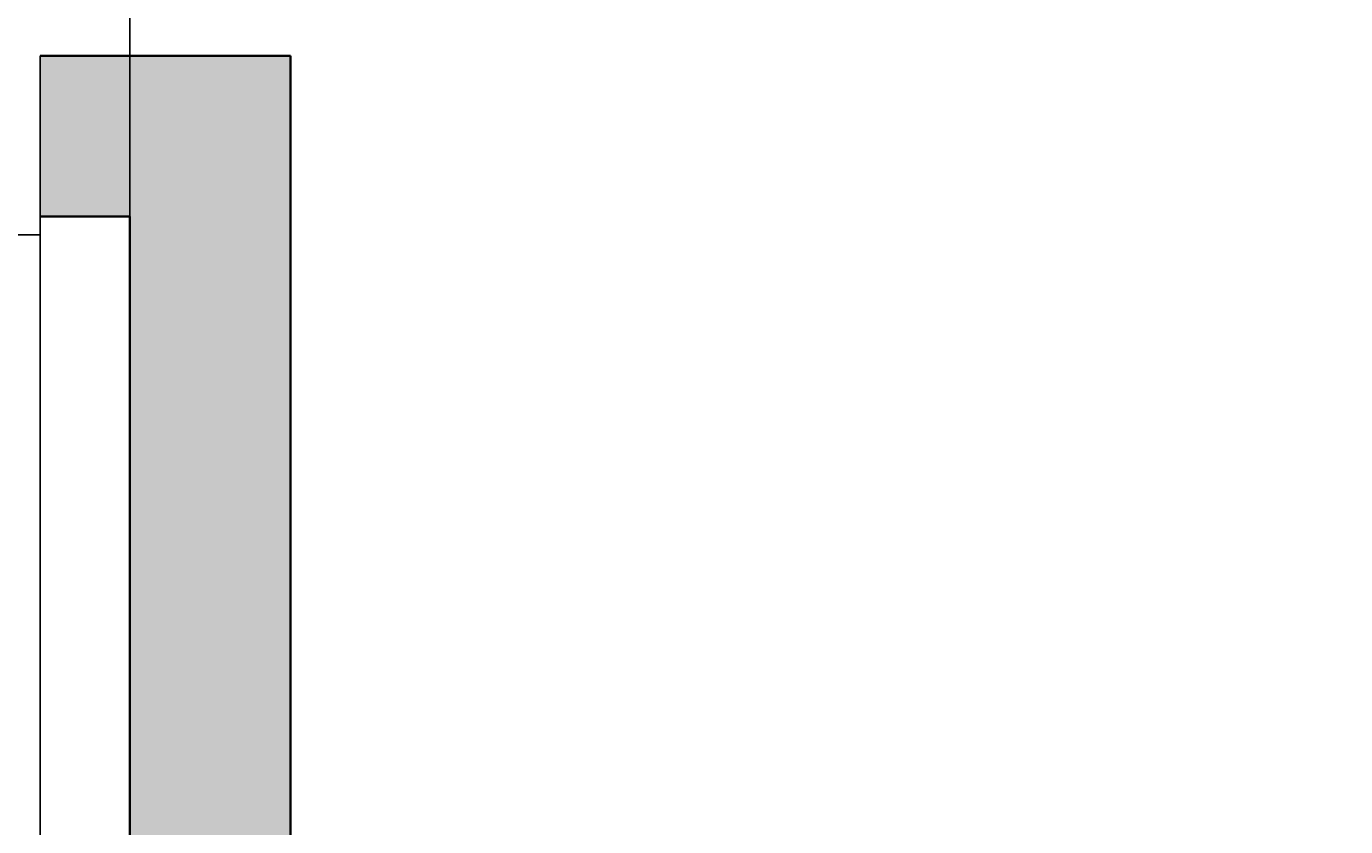
# Model space of a CAD drawing. Units: inches. Extents: x 1998 to 2588, y 1139 to 1977.
# Tile 54 of 134: x 2220 to 2257, y 1686 to 1708. Entities that reach past the tile are written whole.
import ezdxf

# ---------------------------------------------------------------- set-up
doc = ezdxf.new("R2010")
doc.units = ezdxf.units.IN
for name, color, linetype, lineweight in [('A-ANNO-DIMS', 2, 'Continuous', 18), ('A-WALL-PATT', 252, 'Continuous', 13), ('DOOR', 52, 'Continuous', 25), ('WALL', 200, 'Continuous', 35)]:
    doc.layers.add(name, color=color, linetype=linetype, lineweight=lineweight)
doc.styles.get("Standard").update_dxf_attribs({"font": 'arial.ttf'})
doc.dimstyles.get("Standard").update_dxf_attribs({"dimtxt": 0.18, "dimasz": 0.18, "dimexe": 0.18, "dimexo": 0.0625, "dimgap": 0.09, "dimtad": 0, "dimtih": 1, "dimtoh": 1, "dimdec": 4, "dimzin": 0, "dimdsep": 46, "dimtxsty": 'Standard', "dimcen": 0.09, "dimadec": 0, "dimazin": 0, "dimtfac": 1, "dimtdec": 4, "dimtofl": 0, "dimtmove": 0, "dimatfit": 3, "dimfxl": 1, "dimtolj": 1, "dimtzin": 0, "dimarcsym": 0})

# ---------------------------------------------------------------- blocks, each defined once
blk = doc.blocks.new('*U2')
for p, q in [((0, 0), (0, -6)), ((40, 0), (40, -6))]:
    blk.add_line(p, q)
blk.add_lwpolyline([(0, 0), (0, 40), (1.75, 40), (1.75, 0)], close=True)
blk.add_arc((0, 0), 40, 0, 90)
blk = doc.blocks.new('*D36')
at = {"layer": 'A-ANNO-DIMS', "color": 0, "lineweight": -2, "transparency": 16777216}
for p, q in [((2197.45, 1663.309), (2197.45, 1977.362)), ((2197.63, 1977.182), (2209.746, 1977.182)), ((2222.793, 1977.182), (2210.677, 1977.182)), ((2222.973, 1663.309), (2222.973, 1977.362))]:
    blk.add_line(p, q, dxfattribs=at)
at = {"layer": 'A-ANNO-DIMS', "color": 0, "transparency": 16777216}
for points in [[(2197.63, 1977.212), (2197.63, 1977.152), (2197.45, 1977.182)], [(2222.793, 1977.212), (2222.793, 1977.152), (2222.973, 1977.182)]]:
    blk.add_solid(points, dxfattribs=at)
at = {"layer": 'Defpoints', "color": 0, "transparency": 16777216}
for p in [(2222.973, 1977.182), (2197.45, 1663.247), (2222.973, 1663.247)]:
    blk.add_point(p, dxfattribs=at)
at = {"layer": 'A-ANNO-DIMS', "color": 0, "transparency": 16777216, "insert": (2210.211, 1977.182), "char_height": 0.18, "attachment_point": 5}
blk.add_mtext('\\A1;25.523', dxfattribs=at)

msp = doc.modelspace()

# ---------------------------------------------------------------- hatches: boundary and pattern name
at = {"layer": 'A-WALL-PATT'}
h = msp.add_hatch(color=256, dxfattribs=at)
h.dxf.hatch_style = 1
h.paths.add_polyline_path([(2527.4729, 1362.2324), (2510.9729, 1362.2324), (2510.9729, 1357.7324), (2518.4729, 1357.7324), (2518.4729, 1237.7324), (2503.1458, 1237.7324), (2503.1458, 1228.7324), (2527.4729, 1228.7324)])
h.paths.add_polyline_path([(2490.5682, 1362.2324), (2398.4729, 1362.2324), (2398.4729, 1357.7324), (2490.5682, 1357.7324)])
h.paths.add_polyline_path([(2224.9729, 1264.7324), (2222.9729, 1264.7324), (2222.9729, 1232.4125), (2341.4729, 1232.4125), (2341.4729, 1234.4125), (2224.9729, 1234.4125)])
h.paths.add_polyline_path([(2334.5332, 1273.7324), (2264.7638, 1273.7324), (2264.7638, 1269.5611, -0.043659), (2264.3413, 1264.7324), (2334.5332, 1264.7324)])
h.paths.add_polyline_path([(2236.9551, 1273.7324), (2234.4125, 1273.7324), (2234.4125, 1264.7324), (2236.9551, 1264.7324), (2236.9551, 1269.5611)])
h.paths.add_polyline_path([(2222.9729, 1293.2324), (2096.9729, 1293.2324), (2096.9729, 1345.0966), (2087.9729, 1345.0966), (2087.9729, 1284.2324), (2222.9729, 1284.2324), (2222.9729, 1285.137)])
h.paths.add_polyline_path([(2096.9729, 1458.7927), (2087.9729, 1458.7927), (2087.9729, 1417.7324), (2087.9729, 1413.2324), (2096.9729, 1413.2324), (2096.9729, 1417.7324)])
h.paths.add_polyline_path([(2096.9729, 1413.2324), (2087.9729, 1413.2324), (2087.9729, 1365.5012), (2096.9729, 1365.5012), (2096.9729, 1369.3358)])
h.paths.add_polyline_path([(2186.2943, 1417.7324), (2138.6074, 1417.7324), (2096.9729, 1417.7324), (2096.9729, 1413.2324), (2138.6074, 1413.2324), (2186.2943, 1413.2324)])
h.paths.add_polyline_path([(2181.4729, 1465.7324), (2176.9729, 1465.7324), (2176.9729, 1451.6434), (2181.4729, 1451.6434)])
h.paths.add_polyline_path([(2181.4729, 1422.1664), (2176.9729, 1422.1664), (2176.9729, 1417.7324), (2181.4729, 1417.7324)])
h.paths.add_polyline_path([(2063.9729, 1465.7324), (2087.9729, 1465.7324), (2087.9729, 1470.2324), (2059.4729, 1470.2324), (2059.4729, 1413.2324), (2087.9729, 1413.2324), (2087.9729, 1417.7324), (2063.9729, 1417.7324)])
h.paths.add_polyline_path([(2181.4729, 1755.2324), (2176.9729, 1755.2324), (2176.9729, 1748.6798), (2177.0513, 1748.6798), (2181.4729, 1748.6798)])
h.paths.add_polyline_path([(2227.4729, 1707.2324), (2220.4647, 1707.2324), (2220.4647, 1702.7324), (2222.9729, 1702.7324), (2222.9729, 1604.637), (2227.4729, 1604.637)])
h.paths.add_polyline_path([(2114.9729, 1702.7324), (2105.9729, 1702.7324), (2105.9729, 1628.4781, -0.0318759), (2110.1012, 1628.7416), (2114.9729, 1628.7416)])
h.paths.add_polyline_path([(2345.9729, 1739.3278), (2341.4729, 1739.3278), (2341.4729, 1647.5211), (2345.9729, 1647.5211)])
h.paths.add_polyline_path([(2350.6273, 1641.2324), (2345.9729, 1641.2324), (2345.9729, 1636.7324), (2350.6273, 1636.7324), (2350.6273, 1639.8729)])
h.paths.add_polyline_path([(2501.9729, 1641.2324), (2407.9729, 1641.2324), (2392.5005, 1641.2324), (2392.5005, 1639.8729), (2392.5005, 1636.7324), (2501.9729, 1636.7324)])
h.paths.add_polyline_path([(2510.9729, 1755.2324), (2501.9729, 1755.2324), (2501.9729, 1641.2324), (2510.9729, 1641.2324)])
h.paths.add_polyline_path([(2549.1786, 1641.2324), (2522.3775, 1641.2324), (2522.3775, 1636.7324), (2540.1786, 1636.7324), (2540.1786, 1480.7324), (2522.3775, 1480.7324), (2522.3775, 1476.2324), (2549.1786, 1476.2324)])
h.paths.add_polyline_path([(2498.1786, 1594.7324), (2407.9729, 1594.7324), (2407.9729, 1585.7324), (2416.9729, 1585.7324), (2489.1786, 1585.7324), (2489.1786, 1531.7324), (2416.9729, 1531.7324), (2407.9729, 1531.7324), (2407.9729, 1522.7324), (2498.1786, 1522.7324)])
h.paths.add_polyline_path([(2351.6437, 1480.7324), (2345.9729, 1480.7324), (2345.9729, 1476.2324), (2351.6437, 1476.2324), (2351.6437, 1477.5919)])
h.paths.add_polyline_path([(2501.9729, 1480.7324), (2498.1786, 1480.7324), (2407.9729, 1480.7324), (2393.5168, 1480.7324), (2393.5168, 1477.5919), (2393.5168, 1476.2324), (2501.9729, 1476.2324)])

# ---------------------------------------------------------------- linework, layer by layer
at = {"layer": 'WALL'}
for p, q in [((2220.4647, 1707.2324), (2222.9729, 1707.2324)), ((2227.4729, 1707.2324), (2220.4647, 1707.2324)), ((2222.9729, 1707.2324), (2227.4729, 1707.2324)), ((2227.4729, 1707.2324), (2227.4729, 1584.2324)), ((2227.4729, 1702.7324), (2227.4729, 1707.2324)), ((2227.4729, 1702.7324), (2227.4729, 1707.2324)), ((2220.4647, 1702.7324), (2222.9729, 1702.7324)), ((2222.9729, 1702.7324), (2220.4647, 1702.7324)), ((2222.9729, 1702.7324), (2222.9729, 1604.637))]:
    msp.add_line(p, q, dxfattribs=at)

# ---------------------------------------------------------------- block references
at = {"layer": 'DOOR', "xscale": 0.8354643497673233, "yscale": 0.8354643497673233, "zscale": 0.8354643497673233, "rotation": 180}
msp.add_blockref('*U2', (2220.4647, 1702.2196), dxfattribs=at)

# ---------------------------------------------------------------- dimensions: what is measured, and where the dimension line sits
at = {"layer": 'A-ANNO-DIMS'}
dim = msp.add_linear_dim(base=(2222.9729, 1977.1824), p1=(2197.4499, 1663.2466), p2=(2222.9729, 1663.2466), dimstyle='Standard', override={"dimdec": 3, "dimlfac": 1, "dimrnd": 0, "dimzin": 0, "dimdsep": 46, "dimlunit": 2}, dxfattribs=at)
dim.commit()
dim.dimension.update_dxf_attribs({"geometry": '*D36', "text_midpoint": (2210.2114, 1977.1824)})

doc.saveas('drawing.dxf')
